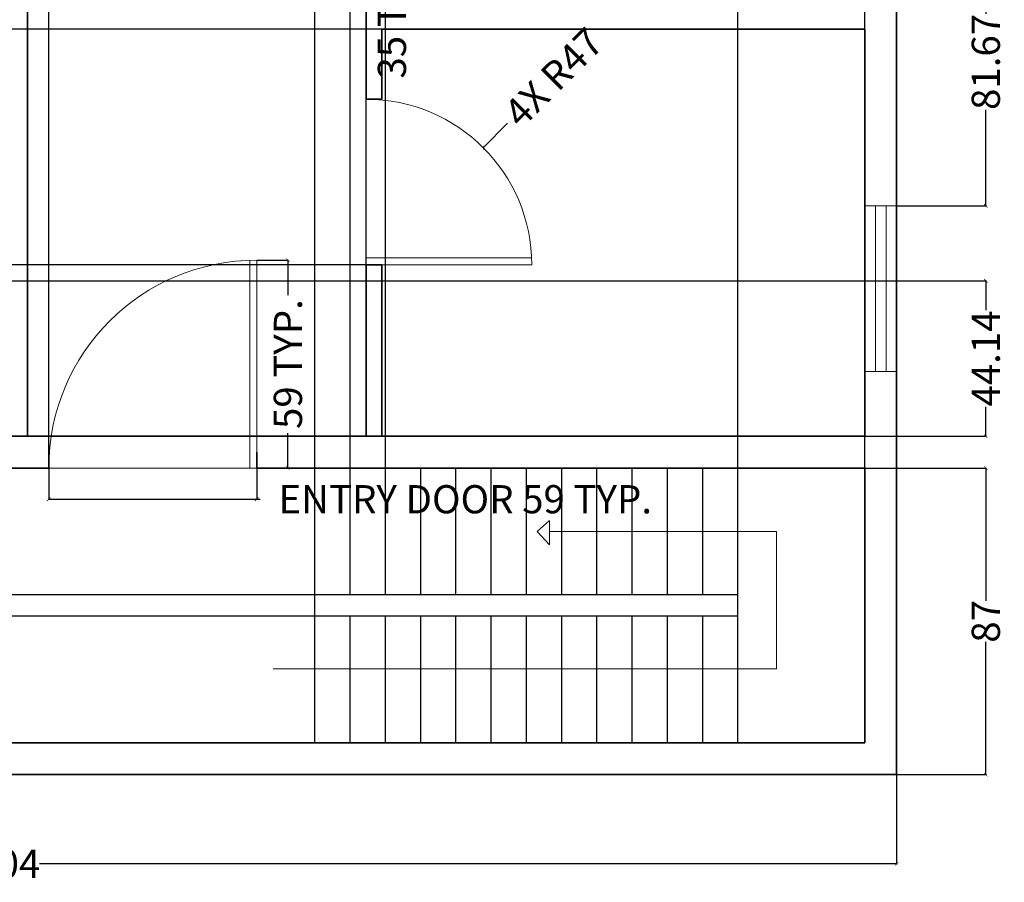
# Model space of a CAD drawing. Units: inches. Extents: x 878 to 1443, y 634 to 1188.
# Tile 4 of 5: x 1164 to 1443, y 634 to 879. Entities that reach past the tile are written whole.
import ezdxf

# ---------------------------------------------------------------- set-up
doc = ezdxf.new("R2010")
doc.units = ezdxf.units.IN
doc.header["$MEASUREMENT"] = 0
for name, color, linetype, lineweight in [('A-ANNO-DIMS', 2, 'Continuous', 18), ('A-FLOR-STRS', 7, 'Continuous', 25), ('A-WALL', 7, 'Continuous', 35)]:
    doc.layers.add(name, color=color, linetype=linetype, lineweight=lineweight)
for name, color, linetype, lineweight, true_color in [('A-ANNO-SYMB', 240, 'Continuous', 18, 0xed1f24), ('A-DOOR', 41, 'Continuous', 18, 0xf4ee51), ('A-GLAZ', 152, 'Continuous', 18, 0x2776bb)]:
    doc.layers.add(name, color=color, linetype=linetype, lineweight=lineweight, true_color=true_color)
doc.styles.get("Standard").update_dxf_attribs({"font": 'arial.ttf'})
doc.dimstyles.get("Standard").update_dxf_attribs({"dimtxt": 8, "dimasz": 1, "dimexe": 0.18, "dimexo": 0.0625, "dimgap": 0.09, "dimtad": 0, "dimdec": 4, "dimzin": 0, "dimdsep": 46, "dimlunit": 3, "dimtxsty": 'Standard', "dimblk": 'ARCHTICK', "dimcen": 0.09, "dimclrd": 6, "dimclre": 5, "dimclrt": 140, "dimadec": 0, "dimazin": 0, "dimtfac": 1, "dimtdec": 4, "dimtofl": 0, "dimtmove": 0, "dimatfit": 3, "dimfxl": 1, "dimtolj": 1, "dimtzin": 0, "dimarcsym": 0})

# ---------------------------------------------------------------- blocks, each defined once
blk = doc.blocks.new('WIN-47IN')
for p, q in [((9, 47), (0, 47)), ((0, 47), (0, 0)), ((3, 0), (3, 47)), ((6, 0), (6, 47)), ((9, 0), (9, 47)), ((0, 0), (9, 0))]:
    blk.add_line(p, q)
blk = doc.blocks.new('DOOR-47IN')
for p, q in [((0, 47), (0, 0)), ((0, 2), (46.96, 2)), ((0, 0), (47, 0))]:
    blk.add_line(p, q)
blk.add_arc((0, 0), 47, 0, 90)
blk = doc.blocks.new('DOOR-59IN')
for p, q in [((57, 0), (57, 58.97)), ((59, 0), (59, 59)), ((0, 0), (59, 0))]:
    blk.add_line(p, q)
blk.add_arc((59, 0), 59, 90, 180)
blk = doc.blocks.new('_ArchTick')
at = {"color": 0, "linetype": 'ByBlock', "const_width": 0.15}
blk.add_lwpolyline([(-0.5, -0.5), (0.5, 0.5)], dxfattribs=at)
blk = doc.blocks.new('*D13')
at = {"layer": 'A-ANNO-DIMS', "color": 5, "lineweight": -2, "transparency": 16777216}
for p, q in [((1172.39, 751.41), (1172.39, 742.44)), ((1231.39, 751.41), (1231.39, 742.44))]:
    blk.add_line(p, q, dxfattribs=at)
at = {"layer": 'A-ANNO-DIMS', "color": 6, "lineweight": -2, "transparency": 16777216}
for p, q in [((1172.39, 742.62), (1231.39, 742.62)), ((1231.39, 742.62), (1232.39, 742.62))]:
    blk.add_line(p, q, dxfattribs=at)
at = {"layer": 'Defpoints', "color": 0, "lineweight": -2, "transparency": 16777216}
for p in [(1172.39, 751.47), (1231.39, 751.47), (1231.39, 742.62)]:
    blk.add_point(p, dxfattribs=at)
at = {"layer": 'A-ANNO-DIMS', "color": 6, "lineweight": -2, "transparency": 16777216, "rotation": 180}
blk.add_blockref('_ArchTick', (1172.39, 742.62), dxfattribs=at)
at = {"layer": 'A-ANNO-DIMS', "color": 6, "lineweight": -2, "transparency": 16777216}
blk.add_blockref('_ArchTick', (1231.39, 742.62), dxfattribs=at)
at = {"layer": 'A-ANNO-DIMS', "color": 140, "transparency": 16777216, "insert": (1290.55, 742.62), "char_height": 8, "attachment_point": 5}
blk.add_mtext('\\A1;ENTRY DOOR 59 TYP.', dxfattribs=at)
blk = doc.blocks.new('*D14')
at = {"layer": 'A-ANNO-DIMS', "color": 5, "lineweight": -2, "transparency": 16777216}
for p, q in [((1231.45, 810.47), (1240.42, 810.47)), ((1231.45, 751.47), (1240.42, 751.47))]:
    blk.add_line(p, q, dxfattribs=at)
at = {"layer": 'A-ANNO-DIMS', "color": 6, "lineweight": -2, "transparency": 16777216}
for p, q in [((1240.24, 810.47), (1240.24, 800.53)), ((1240.24, 751.47), (1240.24, 761.41))]:
    blk.add_line(p, q, dxfattribs=at)
at = {"layer": 'Defpoints', "color": 0, "lineweight": -2, "transparency": 16777216}
for p in [(1231.39, 810.47), (1240.24, 810.47), (1231.39, 751.47)]:
    blk.add_point(p, dxfattribs=at)
at = {"layer": 'A-ANNO-DIMS', "color": 6, "lineweight": -2, "transparency": 16777216}
for p, rotation in [((1240.24, 810.47), 90), ((1240.24, 751.47), 270)]:
    blk.add_blockref('_ArchTick', p, dxfattribs=dict(at, rotation=rotation))
at = {"layer": 'A-ANNO-DIMS', "color": 140, "transparency": 16777216, "insert": (1240.24, 780.97), "char_height": 8, "attachment_point": 5, "rotation": 90}
blk.add_mtext('\\A1;59 TYP.', dxfattribs=at)
blk = doc.blocks.new('*D18')
at = {"layer": 'A-ANNO-DIMS', "color": 5, "lineweight": -2, "transparency": 16777216}
for p, q in [((1274.92, 935.97), (1269.56, 935.97)), ((1274.92, 900.97), (1269.56, 900.97))]:
    blk.add_line(p, q, dxfattribs=at)
at = {"layer": 'A-ANNO-DIMS', "color": 6, "lineweight": -2, "transparency": 16777216}
for p, q in [((1269.74, 935.97), (1269.74, 900.97)), ((1269.74, 900.97), (1269.74, 899.97))]:
    blk.add_line(p, q, dxfattribs=at)
at = {"layer": 'Defpoints', "color": 0, "lineweight": -2, "transparency": 16777216}
for p in [(1274.99, 935.97), (1269.74, 900.97), (1274.99, 900.97)]:
    blk.add_point(p, dxfattribs=at)
at = {"layer": 'A-ANNO-DIMS', "color": 6, "lineweight": -2, "transparency": 16777216}
for p, rotation in [((1269.74, 935.97), 90), ((1269.74, 900.97), 270)]:
    blk.add_blockref('_ArchTick', p, dxfattribs=dict(at, rotation=rotation))
at = {"layer": 'A-ANNO-DIMS', "color": 140, "transparency": 16777216, "insert": (1269.74, 880.41), "char_height": 8, "attachment_point": 5, "rotation": 90}
blk.add_mtext('\\A1;35 TYP.', dxfattribs=at)
blk = doc.blocks.new('*D21')
at = {"layer": 'A-ANNO-DIMS', "color": 5, "lineweight": -2, "transparency": 16777216}
for p, q in [((908.9, 664.41), (908.9, 638.98)), ((1412.9, 664.41), (1412.9, 638.98))]:
    blk.add_line(p, q, dxfattribs=at)
at = {"layer": 'A-ANNO-DIMS', "color": 6, "lineweight": -2, "transparency": 16777216}
for p, q in [((908.9, 639.16), (1151.99, 639.16)), ((1412.9, 639.16), (1169.81, 639.16))]:
    blk.add_line(p, q, dxfattribs=at)
at = {"layer": 'Defpoints', "color": 0, "lineweight": -2, "transparency": 16777216}
for p in [(908.9, 664.47), (1412.9, 664.47), (1412.9, 639.16)]:
    blk.add_point(p, dxfattribs=at)
at = {"layer": 'A-ANNO-DIMS', "color": 6, "lineweight": -2, "transparency": 16777216, "rotation": 180}
blk.add_blockref('_ArchTick', (908.9, 639.16), dxfattribs=at)
at = {"layer": 'A-ANNO-DIMS', "color": 6, "lineweight": -2, "transparency": 16777216}
blk.add_blockref('_ArchTick', (1412.9, 639.16), dxfattribs=at)
at = {"layer": 'A-ANNO-DIMS', "color": 140, "transparency": 16777216, "insert": (1160.9, 639.16), "char_height": 8, "attachment_point": 5}
blk.add_mtext('\\A1;504', dxfattribs=at)
blk = doc.blocks.new('*D23')
at = {"layer": 'A-ANNO-DIMS', "color": 5, "lineweight": -2, "transparency": 16777216}
for p, q in [((1403.96, 751.47), (1438.39, 751.47)), ((1412.96, 664.47), (1438.39, 664.47))]:
    blk.add_line(p, q, dxfattribs=at)
at = {"layer": 'A-ANNO-DIMS', "color": 6, "lineweight": -2, "transparency": 16777216}
for p, q in [((1438.21, 751.47), (1438.21, 713.8)), ((1438.21, 664.47), (1438.21, 702.14))]:
    blk.add_line(p, q, dxfattribs=at)
at = {"layer": 'Defpoints', "color": 0, "lineweight": -2, "transparency": 16777216}
for p in [(1403.9, 751.47), (1438.21, 751.47), (1412.9, 664.47)]:
    blk.add_point(p, dxfattribs=at)
at = {"layer": 'A-ANNO-DIMS', "color": 6, "lineweight": -2, "transparency": 16777216}
for p, rotation in [((1438.21, 751.47), 90), ((1438.21, 664.47), 270)]:
    blk.add_blockref('_ArchTick', p, dxfattribs=dict(at, rotation=rotation))
at = {"layer": 'A-ANNO-DIMS', "color": 140, "transparency": 16777216, "insert": (1438.21, 707.97), "char_height": 8, "attachment_point": 5, "rotation": 90}
blk.add_mtext('\\A1;87', dxfattribs=at)
blk = doc.blocks.new('*D32')
at = {"layer": 'A-ANNO-DIMS', "color": 5, "lineweight": -2, "transparency": 16777216}
for p, q in [((1412.96, 907.55), (1438.39, 907.55)), ((1412.96, 825.89), (1438.39, 825.89))]:
    blk.add_line(p, q, dxfattribs=at)
at = {"layer": 'A-ANNO-DIMS', "color": 6, "lineweight": -2, "transparency": 16777216}
for p, q in [((1438.21, 907.55), (1438.21, 880.32)), ((1438.21, 825.89), (1438.21, 853.13))]:
    blk.add_line(p, q, dxfattribs=at)
at = {"layer": 'Defpoints', "color": 0, "lineweight": -2, "transparency": 16777216}
for p in [(1412.9, 907.55), (1412.9, 825.89), (1438.21, 825.89)]:
    blk.add_point(p, dxfattribs=at)
at = {"layer": 'A-ANNO-DIMS', "color": 6, "lineweight": -2, "transparency": 16777216}
for p, rotation in [((1438.21, 907.55), 90), ((1438.21, 825.89), 270)]:
    blk.add_blockref('_ArchTick', p, dxfattribs=dict(at, rotation=rotation))
at = {"layer": 'A-ANNO-DIMS', "color": 140, "transparency": 16777216, "insert": (1438.21, 866.72), "char_height": 8, "attachment_point": 5, "rotation": 90}
blk.add_mtext('\\A1;81.67', dxfattribs=at)
blk = doc.blocks.new('*D35')
at = {"layer": 'A-ANNO-DIMS', "color": 5, "lineweight": -2, "transparency": 16777216}
for p, q in [((1166.4, 760.53), (1166.4, 1145.96)), ((1262.4, 760.53), (1262.4, 1145.96))]:
    blk.add_line(p, q, dxfattribs=at)
at = {"layer": 'A-ANNO-DIMS', "color": 6, "lineweight": -2, "transparency": 16777216}
for p, q in [((1166.4, 1145.78), (1208.58, 1145.78)), ((1262.4, 1145.78), (1220.22, 1145.78))]:
    blk.add_line(p, q, dxfattribs=at)
at = {"layer": 'Defpoints', "color": 0, "lineweight": -2, "transparency": 16777216}
for p in [(1262.4, 1145.78), (1166.4, 760.47), (1262.4, 760.47)]:
    blk.add_point(p, dxfattribs=at)
at = {"layer": 'A-ANNO-DIMS', "color": 6, "lineweight": -2, "transparency": 16777216, "rotation": 180}
blk.add_blockref('_ArchTick', (1166.4, 1145.78), dxfattribs=at)
at = {"layer": 'A-ANNO-DIMS', "color": 6, "lineweight": -2, "transparency": 16777216}
blk.add_blockref('_ArchTick', (1262.4, 1145.78), dxfattribs=at)
at = {"layer": 'A-ANNO-DIMS', "color": 140, "transparency": 16777216, "insert": (1214.4, 1145.78), "char_height": 8, "attachment_point": 5}
blk.add_mtext('\\A1;96', dxfattribs=at)
blk = doc.blocks.new('*D38')
at = {"layer": 'A-ANNO-DIMS', "color": 5, "lineweight": -2, "transparency": 16777216}
for p, q in [((1403.84, 875.97), (883.41, 875.97)), ((1403.84, 760.47), (883.41, 760.47))]:
    blk.add_line(p, q, dxfattribs=at)
at = {"layer": 'A-ANNO-DIMS', "color": 6, "lineweight": -2, "transparency": 16777216}
for p, q in [((883.59, 875.97), (883.59, 831.46)), ((883.59, 760.47), (883.59, 804.98))]:
    blk.add_line(p, q, dxfattribs=at)
at = {"layer": 'Defpoints', "color": 0, "lineweight": -2, "transparency": 16777216}
for p in [(1403.9, 875.97), (883.59, 760.47), (1403.9, 760.47)]:
    blk.add_point(p, dxfattribs=at)
at = {"layer": 'A-ANNO-DIMS', "color": 6, "lineweight": -2, "transparency": 16777216}
for p, rotation in [((883.59, 875.97), 90), ((883.59, 760.47), 270)]:
    blk.add_blockref('_ArchTick', p, dxfattribs=dict(at, rotation=rotation))
at = {"layer": 'A-ANNO-DIMS', "color": 140, "transparency": 16777216, "insert": (883.59, 818.22), "char_height": 8, "attachment_point": 5, "rotation": 90}
blk.add_mtext('\\A1;115.5', dxfattribs=at)
blk = doc.blocks.new('*D46')
at = {"layer": 'A-ANNO-DIMS', "color": 5, "lineweight": -2, "transparency": 16777216}
for p, q in [((1110.3, 751.53), (1110.3, 1145.96)), ((1172.39, 751.53), (1172.39, 1145.96))]:
    blk.add_line(p, q, dxfattribs=at)
at = {"layer": 'A-ANNO-DIMS', "color": 6, "lineweight": -2, "transparency": 16777216}
for p, q in [((1110.3, 1145.78), (1127.73, 1145.78)), ((1172.39, 1145.78), (1154.96, 1145.78))]:
    blk.add_line(p, q, dxfattribs=at)
at = {"layer": 'Defpoints', "color": 0, "lineweight": -2, "transparency": 16777216}
for p in [(1172.39, 1145.78), (1110.3, 751.47), (1172.39, 751.47)]:
    blk.add_point(p, dxfattribs=at)
at = {"layer": 'A-ANNO-DIMS', "color": 6, "lineweight": -2, "transparency": 16777216, "rotation": 180}
blk.add_blockref('_ArchTick', (1110.3, 1145.78), dxfattribs=at)
at = {"layer": 'A-ANNO-DIMS', "color": 6, "lineweight": -2, "transparency": 16777216}
blk.add_blockref('_ArchTick', (1172.39, 1145.78), dxfattribs=at)
at = {"layer": 'A-ANNO-DIMS', "color": 140, "transparency": 16777216, "insert": (1141.35, 1145.78), "char_height": 8, "attachment_point": 5}
blk.add_mtext('\\A1;62.08', dxfattribs=at)
blk = doc.blocks.new('*D47')
at = {"layer": 'A-ANNO-DIMS', "color": 5, "lineweight": -2, "transparency": 16777216}
for p, q in [((1020.46, 804.61), (1438.39, 804.61)), ((1020.46, 760.47), (1438.39, 760.47))]:
    blk.add_line(p, q, dxfattribs=at)
at = {"layer": 'A-ANNO-DIMS', "color": 6, "lineweight": -2, "transparency": 16777216}
for p, q in [((1438.21, 804.61), (1438.21, 796.27)), ((1438.21, 760.47), (1438.21, 768.81))]:
    blk.add_line(p, q, dxfattribs=at)
at = {"layer": 'Defpoints', "color": 0, "lineweight": -2, "transparency": 16777216}
for p in [(1020.4, 804.61), (1438.21, 804.61), (1020.4, 760.47)]:
    blk.add_point(p, dxfattribs=at)
at = {"layer": 'A-ANNO-DIMS', "color": 6, "lineweight": -2, "transparency": 16777216}
for p, rotation in [((1438.21, 804.61), 90), ((1438.21, 760.47), 270)]:
    blk.add_blockref('_ArchTick', p, dxfattribs=dict(at, rotation=rotation))
at = {"layer": 'A-ANNO-DIMS', "color": 140, "transparency": 16777216, "insert": (1438.21, 782.54), "char_height": 8, "attachment_point": 5, "rotation": 90}
blk.add_mtext('\\A1;44.14', dxfattribs=at)
blk = doc.blocks.new('*D48')
at = {"layer": 'A-ANNO-DIMS', "color": 5, "lineweight": -2, "transparency": 16777216}
for p, q in [((1262.34, 809.15), (883.41, 809.15)), ((1262.34, 760.47), (883.41, 760.47))]:
    blk.add_line(p, q, dxfattribs=at)
at = {"layer": 'A-ANNO-DIMS', "color": 6, "lineweight": -2, "transparency": 16777216}
for p, q in [((883.59, 809.15), (883.59, 798.57)), ((883.59, 760.47), (883.59, 771.05))]:
    blk.add_line(p, q, dxfattribs=at)
at = {"layer": 'Defpoints', "color": 0, "lineweight": -2, "transparency": 16777216}
for p in [(883.59, 809.15), (1262.4, 809.15), (1262.4, 760.47)]:
    blk.add_point(p, dxfattribs=at)
at = {"layer": 'A-ANNO-DIMS', "color": 6, "lineweight": -2, "transparency": 16777216}
for p, rotation in [((883.59, 809.15), 90), ((883.59, 760.47), 270)]:
    blk.add_blockref('_ArchTick', p, dxfattribs=dict(at, rotation=rotation))
at = {"layer": 'A-ANNO-DIMS', "color": 140, "transparency": 16777216, "insert": (883.59, 784.81), "char_height": 8, "attachment_point": 5, "rotation": 90}
blk.add_mtext('\\A1;48.68', dxfattribs=at)
blk = doc.blocks.new('*D58')
at = {"layer": 'A-ANNO-DIMS', "color": 5, "lineweight": -2, "transparency": 16777216}
for p, q in [((1367.9, 673.53), (1367.9, 1145.96)), ((1403.9, 673.53), (1403.9, 1145.96))]:
    blk.add_line(p, q, dxfattribs=at)
at = {"layer": 'A-ANNO-DIMS', "color": 6, "lineweight": -2, "transparency": 16777216}
for p, q in [((1367.9, 1145.78), (1380.08, 1145.78)), ((1403.9, 1145.78), (1391.71, 1145.78))]:
    blk.add_line(p, q, dxfattribs=at)
at = {"layer": 'Defpoints', "color": 0, "lineweight": -2, "transparency": 16777216}
for p in [(1403.9, 1145.78), (1367.9, 673.47), (1403.9, 673.47)]:
    blk.add_point(p, dxfattribs=at)
at = {"layer": 'A-ANNO-DIMS', "color": 6, "lineweight": -2, "transparency": 16777216, "rotation": 180}
blk.add_blockref('_ArchTick', (1367.9, 1145.78), dxfattribs=at)
at = {"layer": 'A-ANNO-DIMS', "color": 6, "lineweight": -2, "transparency": 16777216}
blk.add_blockref('_ArchTick', (1403.9, 1145.78), dxfattribs=at)
at = {"layer": 'A-ANNO-DIMS', "color": 140, "transparency": 16777216, "insert": (1385.9, 1145.78), "char_height": 8, "attachment_point": 5}
blk.add_mtext('\\A1;36', dxfattribs=at)
blk = doc.blocks.new('*D59')
at = {"layer": 'A-ANNO-DIMS', "color": 5, "lineweight": -2, "transparency": 16777216}
for p, q in [((1247.9, 709.53), (1247.9, 1145.96)), ((1367.9, 709.53), (1367.9, 1145.96))]:
    blk.add_line(p, q, dxfattribs=at)
at = {"layer": 'A-ANNO-DIMS', "color": 6, "lineweight": -2, "transparency": 16777216}
for p, q in [((1247.9, 1145.78), (1299.36, 1145.78)), ((1367.9, 1145.78), (1316.44, 1145.78))]:
    blk.add_line(p, q, dxfattribs=at)
at = {"layer": 'Defpoints', "color": 0, "lineweight": -2, "transparency": 16777216}
for p in [(1367.9, 1145.78), (1247.9, 709.47), (1367.9, 709.47)]:
    blk.add_point(p, dxfattribs=at)
at = {"layer": 'A-ANNO-DIMS', "color": 6, "lineweight": -2, "transparency": 16777216, "rotation": 180}
blk.add_blockref('_ArchTick', (1247.9, 1145.78), dxfattribs=at)
at = {"layer": 'A-ANNO-DIMS', "color": 6, "lineweight": -2, "transparency": 16777216}
blk.add_blockref('_ArchTick', (1367.9, 1145.78), dxfattribs=at)
at = {"layer": 'A-ANNO-DIMS', "color": 140, "transparency": 16777216, "insert": (1307.9, 1145.78), "char_height": 8, "attachment_point": 5}
blk.add_mtext('\\A1;120', dxfattribs=at)
blk = doc.blocks.new('*D60')
at = {"layer": 'A-ANNO-DIMS', "color": 5, "lineweight": -2, "transparency": 16777216}
for p, q in [((1247.84, 709.47), (883.41, 709.47)), ((1247.84, 673.47), (883.41, 673.47))]:
    blk.add_line(p, q, dxfattribs=at)
at = {"layer": 'A-ANNO-DIMS', "color": 6, "lineweight": -2, "transparency": 16777216}
for p, q in [((883.59, 709.47), (883.59, 697.28)), ((883.59, 673.47), (883.59, 685.66))]:
    blk.add_line(p, q, dxfattribs=at)
at = {"layer": 'Defpoints', "color": 0, "lineweight": -2, "transparency": 16777216}
for p in [(883.59, 709.47), (1247.9, 709.47), (1247.9, 673.47)]:
    blk.add_point(p, dxfattribs=at)
at = {"layer": 'A-ANNO-DIMS', "color": 6, "lineweight": -2, "transparency": 16777216}
for p, rotation in [((883.59, 709.47), 90), ((883.59, 673.47), 270)]:
    blk.add_blockref('_ArchTick', p, dxfattribs=dict(at, rotation=rotation))
at = {"layer": 'A-ANNO-DIMS', "color": 140, "transparency": 16777216, "insert": (883.59, 691.47), "char_height": 8, "attachment_point": 5, "rotation": 90}
blk.add_mtext('\\A1;36', dxfattribs=at)
blk = doc.blocks.new('*D61')
at = {"layer": 'A-ANNO-DIMS', "color": 5, "lineweight": -2, "transparency": 16777216}
for p, q in [((1247.84, 715.47), (883.41, 715.47)), ((1247.84, 709.47), (883.41, 709.47))]:
    blk.add_line(p, q, dxfattribs=at)
at = {"layer": 'A-ANNO-DIMS', "color": 6, "lineweight": -2, "transparency": 16777216}
for p, q in [((883.59, 715.47), (883.59, 715.2)), ((883.59, 709.47), (883.59, 709.74))]:
    blk.add_line(p, q, dxfattribs=at)
at = {"layer": 'Defpoints', "color": 0, "lineweight": -2, "transparency": 16777216}
for p in [(883.59, 715.47), (1247.9, 715.47), (1247.9, 709.47)]:
    blk.add_point(p, dxfattribs=at)
at = {"layer": 'A-ANNO-DIMS', "color": 6, "lineweight": -2, "transparency": 16777216}
for p, rotation in [((883.59, 715.47), 90), ((883.59, 709.47), 270)]:
    blk.add_blockref('_ArchTick', p, dxfattribs=dict(at, rotation=rotation))
at = {"layer": 'A-ANNO-DIMS', "color": 140, "transparency": 16777216, "insert": (883.59, 712.47), "char_height": 8, "attachment_point": 5, "rotation": 90}
blk.add_mtext('\\A1;6', dxfattribs=at)
blk = doc.blocks.new('*D62')
at = {"layer": 'A-ANNO-DIMS', "color": 5, "lineweight": -2, "transparency": 16777216}
for p, q in [((1257.9, 751.53), (1257.9, 1145.96)), ((1267.9, 751.53), (1267.9, 1145.96))]:
    blk.add_line(p, q, dxfattribs=at)
at = {"layer": 'A-ANNO-DIMS', "color": 6, "lineweight": -2, "transparency": 16777216}
for p, q in [((1257.9, 1145.78), (1267.9, 1145.78)), ((1267.9, 1145.78), (1268.9, 1145.78))]:
    blk.add_line(p, q, dxfattribs=at)
at = {"layer": 'Defpoints', "color": 0, "lineweight": -2, "transparency": 16777216}
for p in [(1267.9, 1145.78), (1257.9, 751.47), (1267.9, 751.47)]:
    blk.add_point(p, dxfattribs=at)
at = {"layer": 'A-ANNO-DIMS', "color": 6, "lineweight": -2, "transparency": 16777216, "rotation": 180}
blk.add_blockref('_ArchTick', (1257.9, 1145.78), dxfattribs=at)
at = {"layer": 'A-ANNO-DIMS', "color": 6, "lineweight": -2, "transparency": 16777216}
blk.add_blockref('_ArchTick', (1267.9, 1145.78), dxfattribs=at)
at = {"layer": 'A-ANNO-DIMS', "color": 140, "transparency": 16777216, "insert": (1274.33, 1145.78), "char_height": 8, "attachment_point": 5}
blk.add_mtext('\\A1;10', dxfattribs=at)
blk = doc.blocks.new('*D69')
at = {"layer": 'A-ANNO-DIMS', "color": 6, "lineweight": -2, "transparency": 16777216}
blk.add_line((1302.56, 849.31), (1295.63, 842.38), dxfattribs=at)
at = {"layer": 'A-ANNO-DIMS', "color": 5, "lineweight": -2, "transparency": 16777216}
for p, q in [((1262.31, 809.15), (1262.49, 809.15)), ((1262.4, 809.06), (1262.4, 809.24))]:
    blk.add_line(p, q, dxfattribs=at)
at = {"layer": 'Defpoints', "color": 0, "lineweight": -2, "transparency": 16777216}
for p in [(1295.63, 842.38), (1262.4, 809.15)]:
    blk.add_point(p, dxfattribs=at)
at = {"layer": 'A-ANNO-DIMS', "color": 6, "lineweight": -2, "transparency": 16777216, "rotation": 225.0001068886206}
blk.add_blockref('_ArchTick', (1295.63, 842.38), dxfattribs=at)
at = {"layer": 'A-ANNO-DIMS', "color": 140, "transparency": 16777216, "insert": (1315.57, 862.32), "char_height": 8, "attachment_point": 5, "rotation": 45.0001}
blk.add_mtext('\\A1;4X R47', dxfattribs=at)

msp = doc.modelspace()

# ---------------------------------------------------------------- linework, layer by layer
at = {"layer": 'A-ANNO-SYMB'}
for p, q in [((1314.4351, 736.6091), (1310.9675, 733.4702)), ((1314.4351, 733.4702), (1314.4351, 736.6091)), ((1310.9675, 733.4702), (1314.4351, 729.6393)), ((1378.8705, 733.4702), (1314.4351, 733.4702)), ((1314.4351, 729.6393), (1314.4351, 733.4702)), ((1378.8705, 694.4702), (1378.8705, 733.4702)), ((1236.0809, 694.4702), (1367.8987, 694.4702)), ((1367.8987, 694.4702), (1378.8705, 694.4702))]:
    msp.add_line(p, q, dxfattribs=at)
at = {"layer": 'A-FLOR-STRS'}
for p, q in [((1257.8987, 715.4702), (1257.8987, 751.4702)), ((1267.8987, 715.4702), (1267.8987, 751.4702)), ((1277.8987, 715.4702), (1277.8987, 751.4702)), ((1287.8987, 715.4702), (1287.8987, 751.4702)), ((1297.8987, 715.4702), (1297.8987, 751.4702)), ((1307.8987, 715.4702), (1307.8987, 751.4702)), ((1317.8987, 715.4702), (1317.8987, 751.4702)), ((1327.8987, 715.4702), (1327.8987, 751.4702)), ((1337.8987, 715.4702), (1337.8987, 751.4702)), ((1347.8987, 715.4702), (1347.8987, 751.4702)), ((1357.8987, 715.4702), (1357.8987, 751.4702)), ((1367.8987, 673.4702), (1367.8987, 751.4702)), ((1247.8987, 673.4702), (1247.8987, 715.4702)), ((1367.8987, 715.4702), (1247.8987, 715.4702)), ((1367.8987, 709.4702), (1247.8987, 709.4702)), ((1257.8987, 673.4702), (1257.8987, 709.4702)), ((1267.8987, 673.4702), (1267.8987, 709.4702)), ((1277.8987, 673.4702), (1277.8987, 709.4702)), ((1287.8987, 673.4702), (1287.8987, 709.4702)), ((1297.8987, 673.4702), (1297.8987, 709.4702)), ((1307.8987, 673.4702), (1307.8987, 709.4702)), ((1317.8987, 673.4702), (1317.8987, 709.4702)), ((1327.8987, 673.4702), (1327.8987, 709.4702)), ((1337.8987, 673.4702), (1337.8987, 709.4702)), ((1347.8987, 673.4702), (1347.8987, 709.4702)), ((1357.8987, 673.4702), (1357.8987, 709.4702))]:
    msp.add_line(p, q, dxfattribs=at)
at = {"layer": 'A-WALL'}
for p, q in [((1412.8987, 1120.4702), (1412.8987, 664.4702)), ((1166.3987, 968.9702), (1166.3987, 760.4702)), ((1262.3987, 935.9702), (1262.3987, 856.1495)), ((1403.8987, 875.9702), (1266.8987, 875.9702)), ((1266.8987, 875.9702), (1266.8987, 856.1495)), ((1403.8987, 875.9702), (1403.8987, 760.4702)), ((1266.8987, 856.1495), (1262.3987, 856.1495)), ((1266.8987, 809.1495), (1262.3987, 809.1495)), ((1262.3987, 809.1495), (1262.3987, 760.4702)), ((1266.8987, 809.1495), (1266.8987, 760.4702)), ((1172.3876, 760.4702), (1166.3987, 760.4702)), ((1262.3987, 760.4702), (1231.3876, 760.4702)), ((1403.8987, 760.4702), (1266.8987, 760.4702)), ((1172.3876, 751.4702), (1172.3876, 755.9702)), ((1231.3876, 751.4702), (1231.3876, 755.9702)), ((1172.3876, 751.4702), (992.0853, 751.4702)), ((1403.8987, 751.4702), (1231.3876, 751.4702)), ((1403.8987, 751.4702), (1403.8987, 673.4702)), ((1403.8987, 673.4702), (917.8987, 673.4702)), ((1412.8987, 664.4702), (908.8987, 664.4702))]:
    msp.add_line(p, q, dxfattribs=at)

# ---------------------------------------------------------------- block references
at = {"layer": 'A-DOOR'}
for name, p in [('DOOR-47IN', (1262.3987, 809.1495)), ('DOOR-59IN', (1172.3876, 751.4702))]:
    msp.add_blockref(name, p, dxfattribs=at)
at = {"layer": 'A-GLAZ'}
msp.add_blockref('WIN-47IN', (1403.8987, 778.8894), dxfattribs=at)

# ---------------------------------------------------------------- dimensions: what is measured, and where the dimension line sits
at = {"layer": 'A-ANNO-DIMS'}
for base, p1, p2, override, picture, middle in [((1172.3876, 1145.7802), (1110.3038, 751.4702), (1172.3876, 751.4702), {"dimdec": 2, "dimlfac": 1, "dimrnd": 0, "dimzin": 0, "dimdsep": 46, "dimlunit": 2}, '*D46', (1141.3457, 1145.7802)), ((1262.3987, 1145.7802), (1166.3987, 760.4702), (1262.3987, 760.4702), {"dimdec": 0, "dimlfac": 1, "dimrnd": 0, "dimzin": 0, "dimdsep": 46, "dimlunit": 2}, '*D35', (1214.3987, 1145.7802)), ((1367.8987, 1145.7802), (1247.8987, 709.4702), (1367.8987, 709.4702), {"dimdec": 0, "dimlfac": 1, "dimrnd": 0, "dimzin": 0, "dimdsep": 46, "dimlunit": 2}, '*D59', (1307.8987, 1145.7802)), ((1267.8987, 1145.7802), (1257.8987, 751.4702), (1267.8987, 751.4702), {"dimdec": 0, "dimlfac": 1, "dimrnd": 0, "dimzin": 0, "dimdsep": 46, "dimlunit": 2}, '*D62', (1274.3284, 1145.7802)), ((1403.8987, 1145.7802), (1367.8987, 673.4702), (1403.8987, 673.4702), {"dimdec": 0, "dimlfac": 1, "dimrnd": 0, "dimzin": 0, "dimdsep": 46, "dimlunit": 2}, '*D58', (1385.8987, 1145.7802)), ((1412.8987, 639.1602), (908.8987, 664.4702), (1412.8987, 664.4702), {"dimdec": 0, "dimlfac": 1, "dimrnd": 0, "dimzin": 0, "dimdsep": 46, "dimlunit": 2}, '*D21', (1160.8987, 639.1602))]:
    dim = msp.add_linear_dim(base=base, p1=p1, p2=p2, dimstyle='Standard', override=override, dxfattribs=at)
    dim.commit()
    dim.dimension.update_dxf_attribs({"geometry": picture, "text_midpoint": middle})
for base, p1, p2, angle, picture, middle in [((1269.7372, 900.9702), (1274.9872, 935.9702), (1274.9872, 900.9702), 270, '*D18', (1269.7372, 880.4123)), ((1240.2376, 810.4702), (1231.3876, 751.4702), (1231.3876, 810.4702), 90, '*D14', (1240.2376, 780.9702))]:
    dim = msp.add_linear_dim(base=base, p1=p1, p2=p2, angle=angle, text='<> TYP.', dimstyle='Standard', override={"dimdec": 0, "dimlfac": 1, "dimrnd": 0, "dimzin": 0, "dimdsep": 46, "dimlunit": 2}, dxfattribs=at)
    dim.commit()
    dim.dimension.update_dxf_attribs({"geometry": picture, "text_midpoint": middle})
for base, p1, p2, override, picture, middle in [((1438.2087, 825.8894), (1412.8987, 907.5545), (1412.8987, 825.8894), {"dimdec": 2, "dimlfac": 1, "dimrnd": 0, "dimzin": 0, "dimdsep": 46, "dimlunit": 2}, '*D32', (1438.2087, 866.722)), ((883.5887, 760.4702), (1403.8987, 875.9702), (1403.8987, 760.4702), {"dimdec": 1, "dimlfac": 1, "dimrnd": 0, "dimzin": 0, "dimdsep": 46, "dimlunit": 2}, '*D38', (883.5887, 818.2202)), ((883.5887, 809.1495), (1262.3987, 760.4702), (1262.3987, 809.1495), {"dimdec": 2, "dimlfac": 1, "dimrnd": 0, "dimzin": 0, "dimdsep": 46, "dimlunit": 2}, '*D48', (883.5887, 784.8099)), ((1438.2087, 804.6074), (1020.3987, 760.4702), (1020.3987, 804.6074), {"dimdec": 2, "dimlfac": 1, "dimrnd": 0, "dimzin": 0, "dimdsep": 46, "dimlunit": 2}, '*D47', (1438.2087, 782.5388)), ((1438.2087, 751.4702), (1412.8987, 664.4702), (1403.8987, 751.4702), {"dimdec": 0, "dimlfac": 1, "dimrnd": 0, "dimzin": 0, "dimdsep": 46, "dimlunit": 2}, '*D23', (1438.2087, 707.9702)), ((883.5887, 715.4702), (1247.8987, 709.4702), (1247.8987, 715.4702), {"dimdec": 0, "dimlfac": 1, "dimrnd": 0, "dimzin": 0, "dimdsep": 46, "dimlunit": 2}, '*D61', (883.5887, 712.4702)), ((883.5887, 709.4702), (1247.8987, 673.4702), (1247.8987, 709.4702), {"dimdec": 0, "dimlfac": 1, "dimrnd": 0, "dimzin": 0, "dimdsep": 46, "dimlunit": 2}, '*D60', (883.5887, 691.4702))]:
    dim = msp.add_linear_dim(base=base, p1=p1, p2=p2, angle=90, dimstyle='Standard', override=override, dxfattribs=at)
    dim.commit()
    dim.dimension.update_dxf_attribs({"geometry": picture, "text_midpoint": middle})
dim = msp.add_radius_dim(center=(1262.3987, 809.1495), mpoint=(1295.6326, 842.3836), text='4X <>', dimstyle='Standard', override={"dimdec": 0, "dimlfac": 1, "dimrnd": 0, "dimzin": 0, "dimdsep": 46, "dimlunit": 2}, dxfattribs=at)
dim.commit()
dim.dimension.update_dxf_attribs({"geometry": '*D69', "text_midpoint": (1315.573, 862.3241), "dimtype": 164})
dim = msp.add_linear_dim(base=(1231.3876, 742.6202), p1=(1172.3876, 751.4702), p2=(1231.3876, 751.4702), text='ENTRY DOOR <> TYP.', dimstyle='Standard', override={"dimdec": 0, "dimlfac": 1, "dimrnd": 0, "dimzin": 0, "dimdsep": 46, "dimlunit": 2}, dxfattribs=at)
dim.commit()
dim.dimension.update_dxf_attribs({"geometry": '*D13', "text_midpoint": (1290.5458, 742.6202)})

doc.saveas('drawing.dxf')
